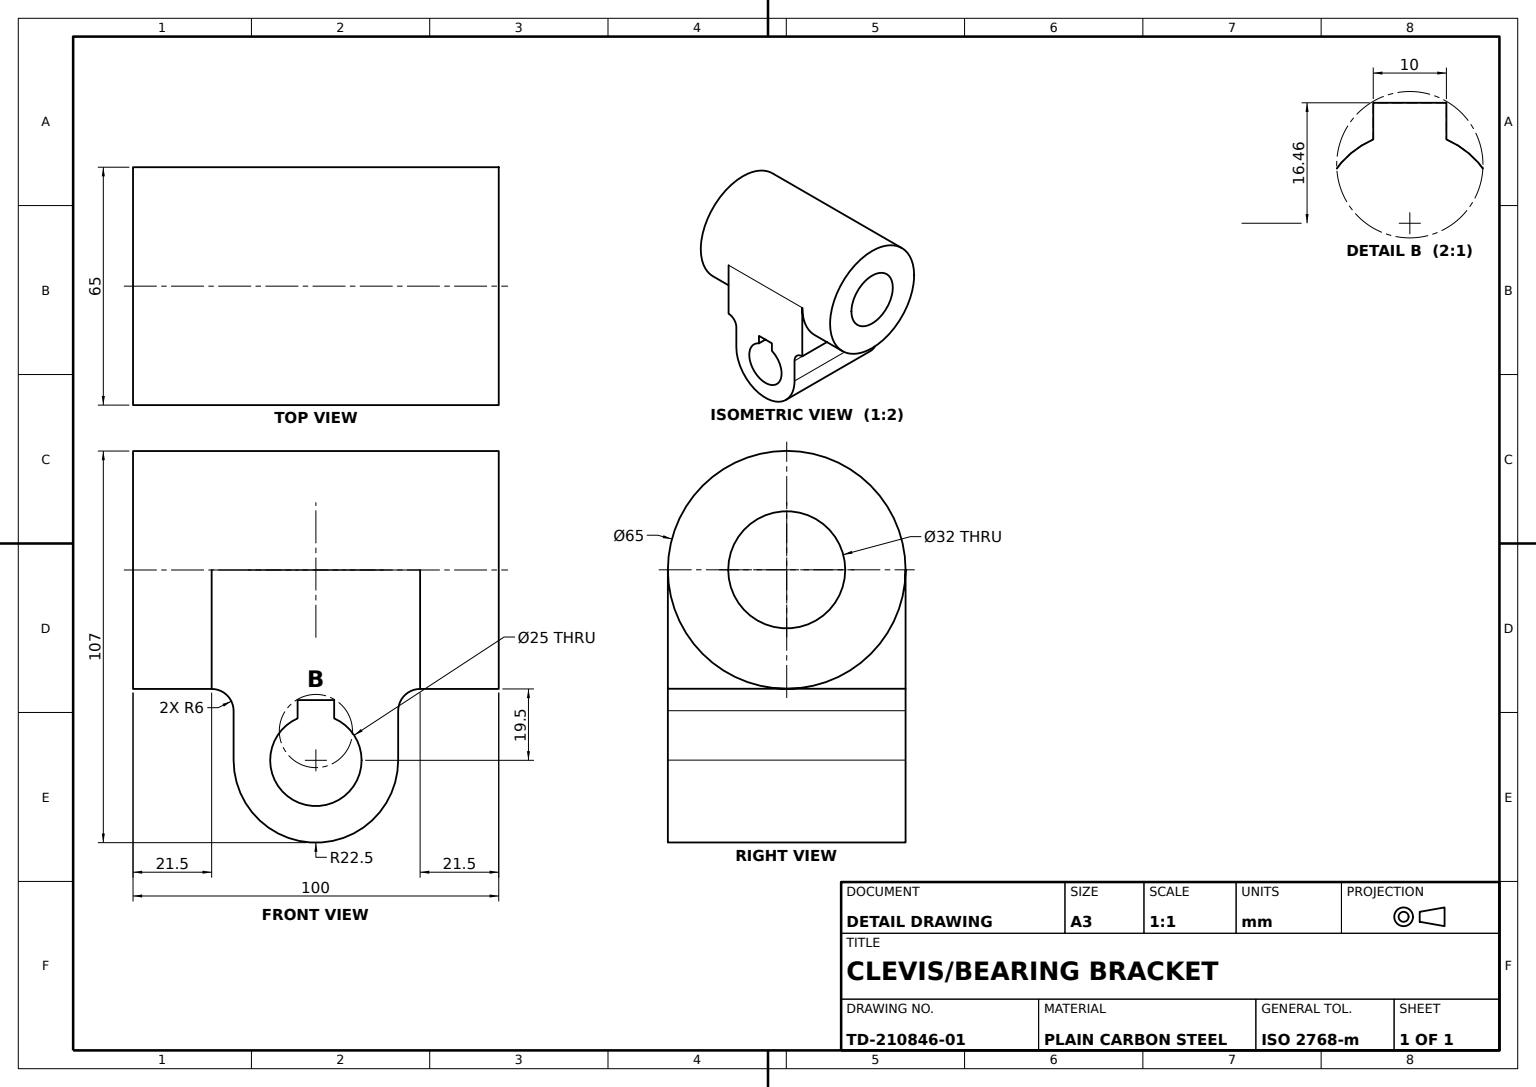
from build123d import *

# Parameters (mm, degrees)
SLEEVE_PROFILE_65_32_R   = 32.5
SLEEVE_PROFILE_65_32_R_2 = 16
SLEEVE_65X100_DEPTH      = 50
BRACKET_WEB_DEPTH        = 32.5
SIDE_RAILS_DEPTH         = 65
LUG_START                = -255
LUG_HOLE_PROFILE_R       = 16
LUG_HOLE_THROUGH_DEPTH   = 255


with BuildPart() as part:
    # Sleeve Profile Ø65-Ø32 → Sleeve Ø65x100 (new, symmetric)
    with BuildSketch(Plane(origin=(0, 0, 0), x_dir=(0, 0, -1), z_dir=(1, 0, 0))):
        Circle(SLEEVE_PROFILE_65_32_R)
        Circle(SLEEVE_PROFILE_65_32_R_2, mode=Mode.SUBTRACT)
    extrude(amount=SLEEVE_65X100_DEPTH, both=True)



with BuildPart() as body_2:
    # Bracket Web Profile → Bracket Web (new, symmetric)
    with BuildSketch(Plane.XY):
        with BuildLine():
            Line((0, -32.5), (-28.5, -32.5))
            ThreePointArc((-28.5, -32.5), (-24.257359313, -34.257359313), (-22.5, -38.5))
            Line((-22.5, -38.5), (-22.5, -52))
            ThreePointArc((-22.5, -52), (0, -74.5), (22.5, -52))
            Line((22.5, -52), (22.5, -38.5))
            ThreePointArc((22.5, -38.5), (24.257359313, -34.257359313), (28.5, -32.5))
            Line((28.5, -32.5), (0, -32.5))
        make_face()
        with BuildLine():
            Line((-5, -35.543560763), (0, -35.543560763))
            Line((0, -35.543560763), (5, -35.543560763))
            Line((5, -35.543560763), (5, -40.543560763))
            ThreePointArc((5, -40.543560763), (0, -64.5), (-5, -40.543560763))
            Line((-5, -40.543560763), (-5, -35.543560763))
        make_face(mode=Mode.SUBTRACT)
    extrude(amount=BRACKET_WEB_DEPTH, both=True)


with BuildPart() as part_1:
    add(part.part)

    add(body_2.part)  # Side Rails merges body 2
    # Side Rail Profile → Side Rails (add)
    # profile 1 of 9: a face of its own
    with BuildSketch(Plane.XY.offset(32.5)):
        with BuildLine():
            Line((-22.5, -32.5), (-28.5, -32.5))
            ThreePointArc((-28.5, -32.5), (-24.257359313, -34.257359313), (-22.5, -38.5))
            Line((-22.5, -38.5), (-22.5, -32.5))
        make_face()
    # profile 2 of 9: a face of its own
    with BuildSketch(Plane.XY.offset(32.5)):
        with BuildLine():
            Line((-23.44711749, -7.891120858), (-28.5, 0))
            Line((-28.5, 0), (-28.5, -32.5))
            Line((-28.5, -32.5), (-22.5, -32.5))
            Line((-22.5, -32.5), (-22.5, -11.126608201))
            ThreePointArc((-22.5, -11.126608201), (-22.741645415, -9.440977022), (-23.44711749, -7.891120858))
        make_face()
    # profile 3 of 9: a face of its own
    with BuildSketch(Plane.XY.offset(32.5)):
        with BuildLine():
            Line((28.5, 0), (-28.5, 0))
            Line((-28.5, 0), (-23.44711749, -7.891120858))
            ThreePointArc((-23.44711749, -7.891120858), (-22.741645415, -9.440977022), (-22.5, -11.126608201))
            Line((-22.5, -11.126608201), (-22.5, -32.5))
            Line((-22.5, -32.5), (-11.22497216, -32.5))
            ThreePointArc((-11.22497216, -32.5), (0, -29.5), (11.22497216, -32.5))
            Line((11.22497216, -32.5), (22.5, -32.5))
            Line((22.5, -32.5), (22.5, -11.126608201))
            ThreePointArc((22.5, -11.126608201), (22.741645415, -9.440977022), (23.44711749, -7.891120858))
            Line((23.44711749, -7.891120858), (28.5, 0))
        make_face()
    # profile 4 of 9: a face of its own
    with BuildSketch(Plane.XY.offset(32.5)):
        with BuildLine():
            Line((28.5, -32.5), (28.5, 0))
            Line((28.5, 0), (23.44711749, -7.891120858))
            ThreePointArc((23.44711749, -7.891120858), (22.741645415, -9.440977022), (22.5, -11.126608201))
            Line((22.5, -11.126608201), (22.5, -32.5))
            Line((22.5, -32.5), (28.5, -32.5))
        make_face()
    # profile 5 of 9: a face of its own
    with BuildSketch(Plane.XY.offset(32.5)):
        with BuildLine():
            Line((22.5, -52), (22.5, -38.5))
            Line((22.5, -38.5), (22.5, -32.5))
            Line((22.5, -32.5), (11.22497216, -32.5))
            ThreePointArc((11.22497216, -32.5), (19.47834533, -40.737493032), (22.5, -52))
        make_face()
    # profile 6 of 9: a face of its own
    with BuildSketch(Plane.XY.offset(32.5)):
        with BuildLine():
            ThreePointArc((22.5, -38.5), (24.257359313, -34.257359313), (28.5, -32.5))
            Line((28.5, -32.5), (22.5, -32.5))
            Line((22.5, -32.5), (22.5, -38.5))
        make_face()
    # profile 7 of 9: a face of its own
    with BuildSketch(Plane.XY.offset(32.5)):
        with BuildLine():
            Line((-22.5, -32.5), (-22.5, -38.5))
            Line((-22.5, -38.5), (-22.5, -52))
            ThreePointArc((-22.5, -52), (-19.47834533, -40.737493032), (-11.22497216, -32.5))
            Line((-11.22497216, -32.5), (-22.5, -32.5))
        make_face()
    # profile 8 of 9: a face of its own
    with BuildSketch(Plane.XY.offset(32.5)):
        with BuildLine():
            ThreePointArc((-11.22497216, -32.5), (-19.47834533, -40.737493032), (-22.5, -52))
            ThreePointArc((-22.5, -52), (0, -74.5), (22.5, -52))
            ThreePointArc((22.5, -52), (19.47834533, -40.737493032), (11.22497216, -32.5))
            Line((11.22497216, -32.5), (-11.22497216, -32.5))
        make_face()
        with BuildLine():
            ThreePointArc((5, -40.543560763), (0, -64.5), (-5, -40.543560763))
            Line((-5, -40.543560763), (-5, -35.543560763))
            Line((-5, -35.543560763), (5, -35.543560763))
            Line((5, -35.543560763), (5, -40.543560763))
        make_face(mode=Mode.SUBTRACT)
    # profile 9 of 9: a face of its own
    with BuildSketch(Plane.XY.offset(32.5)):
        with BuildLine():
            ThreePointArc((11.22497216, -32.5), (0, -29.5), (-11.22497216, -32.5))
            Line((-11.22497216, -32.5), (11.22497216, -32.5))
        make_face()
    extrude(amount=-SIDE_RAILS_DEPTH)

    # Lug Hole Profile → Lug Hole Through (cut)
    with BuildSketch(Plane(origin=(50, 0, 0), x_dir=(0, 0, -1), z_dir=(1, 0, 0)).offset(LUG_START)):
        Circle(LUG_HOLE_PROFILE_R)
    extrude(amount=LUG_HOLE_THROUGH_DEPTH, mode=Mode.SUBTRACT)


solid = part_1.part
